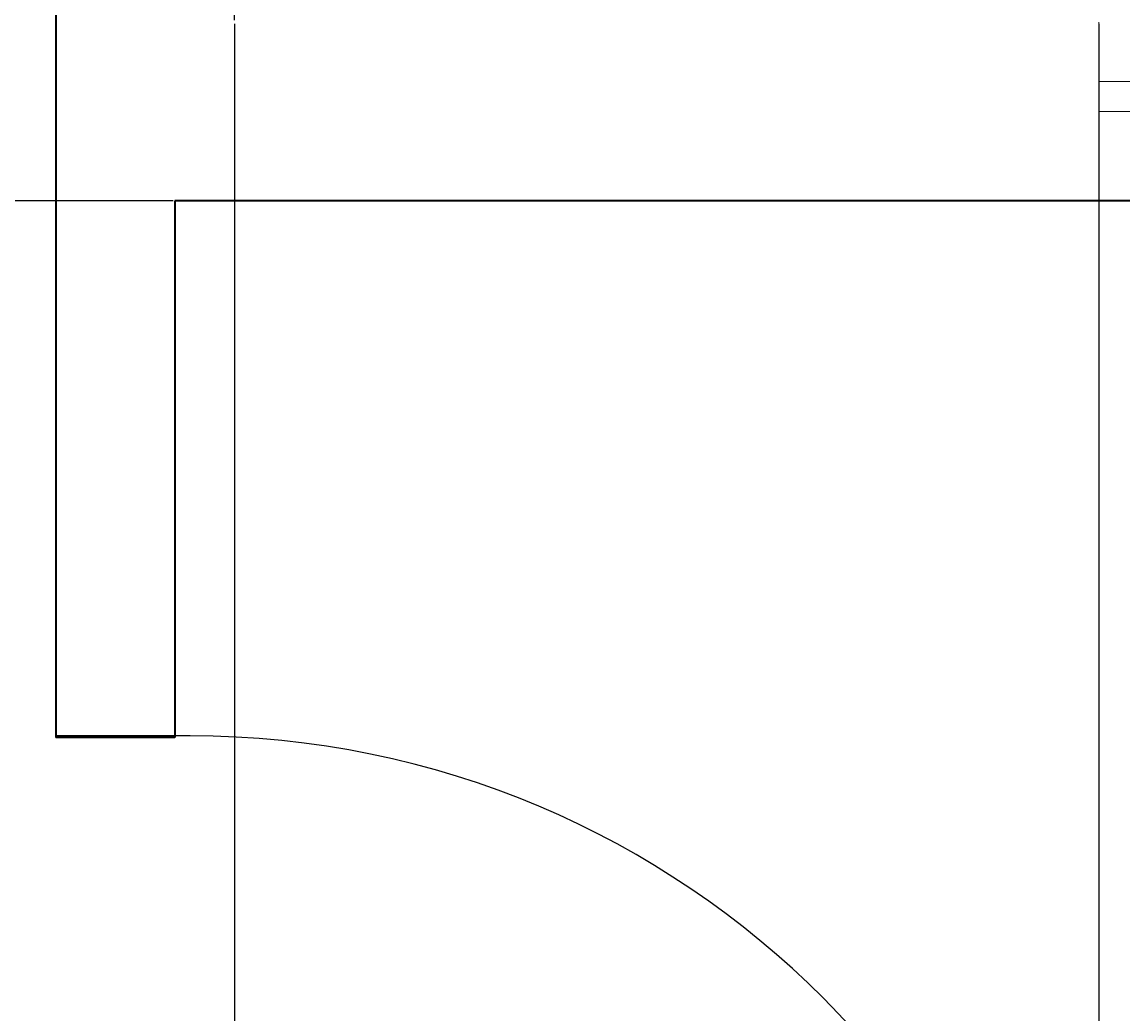
# Model space of a CAD drawing. Units: feet. Extents: x 105 to 1094, y -88 to 588.
# Tile 8 of 59: x 288 to 324, y 171 to 204. Entities that reach past the tile are written whole.
import ezdxf

# ---------------------------------------------------------------- set-up
doc = ezdxf.new("R2010")
doc.units = ezdxf.units.FT
doc.header["$MEASUREMENT"] = 0
for name, color, linetype, lineweight in [('A-ANNO-DIMS', 2, 'Continuous', 18), ('A-DOOR', 3, 'Continuous', 25), ('A-GLAZ', 4, 'Continuous', 18), ('A-WALL', 7, 'Continuous', 35)]:
    doc.layers.add(name, color=color, linetype=linetype, lineweight=lineweight)
doc.styles.get("Standard").update_dxf_attribs({"font": 'arial.ttf'})
doc.dimstyles.get("Standard").update_dxf_attribs({"dimtxt": 0.18, "dimasz": 0.18, "dimexe": 0.18, "dimexo": 0.0625, "dimgap": 0.09, "dimtad": 0, "dimtih": 1, "dimtoh": 1, "dimdec": 4, "dimzin": 0, "dimdsep": 46, "dimtxsty": 'Standard', "dimcen": 0.09, "dimadec": 0, "dimazin": 0, "dimtfac": 1, "dimtdec": 4, "dimtofl": 0, "dimtmove": 0, "dimatfit": 3, "dimfxl": 1, "dimtolj": 1, "dimtzin": 0, "dimarcsym": 0})

# ---------------------------------------------------------------- blocks, each defined once
blk = doc.blocks.new('*U4')
for p, q in [((0, 0), (0, -6)), ((-40, 0), (-40, -6))]:
    blk.add_line(p, q)
blk.add_lwpolyline([(0, 0), (0, 40), (-1.75, 40), (-1.75, 0)], close=True)
blk.add_arc((0, 0), 40, 90, 180)
blk = doc.blocks.new('VENT-TRANSVERSE')
for p, q in [((0, 0), (0, 6)), ((18, 0), (18, 6)), ((0, 3), (18, 3)), ((0, 2), (18, 2))]:
    blk.add_line(p, q)
blk = doc.blocks.new('*D20')
at = {"layer": 'A-ANNO-DIMS', "color": 0, "lineweight": -2, "transparency": 16777216}
for p, q in [((150.688, 276.019), (150.688, -88.149)), ((1048.688, 276.019), (1048.688, -88.149)), ((150.868, -87.969), (599.399, -87.969)), ((1048.508, -87.969), (599.977, -87.969))]:
    blk.add_line(p, q, dxfattribs=at)
at = {"layer": 'A-ANNO-DIMS', "color": 0, "transparency": 16777216}
for points in [[(150.868, -87.939), (150.868, -87.999), (150.688, -87.969)], [(1048.508, -87.939), (1048.508, -87.999), (1048.688, -87.969)]]:
    blk.add_solid(points, dxfattribs=at)
at = {"layer": 'Defpoints', "color": 0, "transparency": 16777216}
for p in [(150.688, 276.081), (1048.688, 276.081), (1048.688, -87.969)]:
    blk.add_point(p, dxfattribs=at)
at = {"layer": 'A-ANNO-DIMS', "color": 0, "transparency": 16777216, "insert": (599.688, -87.969), "char_height": 0.18, "attachment_point": 5}
blk.add_mtext('\\A1;898', dxfattribs=at)
blk = doc.blocks.new('*D21')
at = {"layer": 'A-ANNO-DIMS', "color": 0, "lineweight": -2, "transparency": 16777216}
for p, q in [((849.626, 543.081), (105.458, 543.081)), ((105.638, 542.901), (105.638, 250.263)), ((105.638, -42.739), (105.638, 249.899)), ((849.626, -42.919), (105.458, -42.919))]:
    blk.add_line(p, q, dxfattribs=at)
at = {"layer": 'A-ANNO-DIMS', "color": 0, "transparency": 16777216}
for points in [[(105.608, 542.901), (105.668, 542.901), (105.638, 543.081)], [(105.608, -42.739), (105.668, -42.739), (105.638, -42.919)]]:
    blk.add_solid(points, dxfattribs=at)
at = {"layer": 'Defpoints', "color": 0, "transparency": 16777216}
for p in [(105.638, 543.081), (849.688, 543.081), (849.688, -42.919)]:
    blk.add_point(p, dxfattribs=at)
at = {"layer": 'A-ANNO-DIMS', "color": 0, "transparency": 16777216, "insert": (105.638, 250.081), "char_height": 0.18, "attachment_point": 5}
blk.add_mtext('\\A1;586', dxfattribs=at)
blk = doc.blocks.new('*D39')
at = {"layer": 'A-ANNO-DIMS', "color": 0, "lineweight": -2, "transparency": 16777216}
for p, q in [((294.688, 204.144), (294.688, 588.311)), ((294.868, 588.131), (332.47, 588.131)), ((370.508, 588.131), (332.906, 588.131)), ((370.688, 204.144), (370.688, 588.311))]:
    blk.add_line(p, q, dxfattribs=at)
at = {"layer": 'A-ANNO-DIMS', "color": 0, "transparency": 16777216}
for points in [[(294.868, 588.161), (294.868, 588.101), (294.688, 588.131)], [(370.508, 588.161), (370.508, 588.101), (370.688, 588.131)]]:
    blk.add_solid(points, dxfattribs=at)
at = {"layer": 'Defpoints', "color": 0, "transparency": 16777216}
for p in [(370.688, 588.131), (294.688, 204.081), (370.688, 204.081)]:
    blk.add_point(p, dxfattribs=at)
at = {"layer": 'A-ANNO-DIMS', "color": 0, "transparency": 16777216, "insert": (332.688, 588.131), "char_height": 0.18, "attachment_point": 5}
blk.add_mtext('\\A1;76', dxfattribs=at)
blk = doc.blocks.new('*D44')
at = {"layer": 'A-ANNO-DIMS', "color": 0, "lineweight": -2, "transparency": 16777216}
for p, q in [((294.688, 204.019), (294.688, -88.149)), ((323.688, 204.019), (323.688, -88.149)), ((294.868, -87.969), (308.968, -87.969)), ((323.508, -87.969), (309.409, -87.969))]:
    blk.add_line(p, q, dxfattribs=at)
at = {"layer": 'A-ANNO-DIMS', "color": 0, "transparency": 16777216}
for points in [[(294.868, -87.939), (294.868, -87.999), (294.688, -87.969)], [(323.508, -87.939), (323.508, -87.999), (323.688, -87.969)]]:
    blk.add_solid(points, dxfattribs=at)
at = {"layer": 'Defpoints', "color": 0, "transparency": 16777216}
for p in [(294.688, 204.081), (323.688, 204.081), (323.688, -87.969)]:
    blk.add_point(p, dxfattribs=at)
at = {"layer": 'A-ANNO-DIMS', "color": 0, "transparency": 16777216, "insert": (309.188, -87.969), "char_height": 0.18, "attachment_point": 5}
blk.add_mtext('\\A1;29', dxfattribs=at)
blk = doc.blocks.new('*D46')
at = {"layer": 'A-ANNO-DIMS', "color": 0, "lineweight": -2, "transparency": 16777216}
for p, q in [((580.626, 206.081), (105.458, 206.081)), ((105.638, 205.901), (105.638, 173.263)), ((105.638, 140.261), (105.638, 172.899)), ((580.626, 140.081), (105.458, 140.081))]:
    blk.add_line(p, q, dxfattribs=at)
at = {"layer": 'A-ANNO-DIMS', "color": 0, "transparency": 16777216}
for points in [[(105.608, 205.901), (105.668, 205.901), (105.638, 206.081)], [(105.608, 140.261), (105.668, 140.261), (105.638, 140.081)]]:
    blk.add_solid(points, dxfattribs=at)
at = {"layer": 'Defpoints', "color": 0, "transparency": 16777216}
for p in [(580.688, 206.081), (105.638, 140.081), (580.688, 140.081)]:
    blk.add_point(p, dxfattribs=at)
at = {"layer": 'A-ANNO-DIMS', "color": 0, "transparency": 16777216, "insert": (105.638, 173.081), "char_height": 0.18, "attachment_point": 5}
blk.add_mtext('\\A1;66', dxfattribs=at)
blk = doc.blocks.new('*D55')
at = {"layer": 'A-ANNO-DIMS', "color": 0, "lineweight": -2, "transparency": 16777216}
for p, q in [((292.626, 198.081), (105.458, 198.081)), ((105.638, 197.901), (105.638, 174.263)), ((105.638, 150.261), (105.638, 173.899)), ((293.134, 150.081), (105.458, 150.081))]:
    blk.add_line(p, q, dxfattribs=at)
at = {"layer": 'A-ANNO-DIMS', "color": 0, "transparency": 16777216}
for points in [[(105.608, 197.901), (105.668, 197.901), (105.638, 198.081)], [(105.608, 150.261), (105.668, 150.261), (105.638, 150.081)]]:
    blk.add_solid(points, dxfattribs=at)
at = {"layer": 'Defpoints', "color": 0, "transparency": 16777216}
for p in [(105.638, 198.081), (292.688, 198.081), (293.197, 150.081)]:
    blk.add_point(p, dxfattribs=at)
at = {"layer": 'A-ANNO-DIMS', "color": 0, "transparency": 16777216, "insert": (105.638, 174.081), "char_height": 0.18, "attachment_point": 5}
blk.add_mtext('\\A1;48', dxfattribs=at)

msp = doc.modelspace()

# ---------------------------------------------------------------- linework, layer by layer
at = {"layer": 'A-WALL'}
for p, q in [((288.6883, 218.0812), (288.6883, 180.0812)), ((370.6883, 198.0812), (292.6883, 198.0812)), ((292.6883, 198.0812), (292.6883, 180.0812)), ((292.6883, 180.0812), (288.6883, 180.0812))]:
    msp.add_line(p, q, dxfattribs=at)

# ---------------------------------------------------------------- block references
at = {"layer": 'A-DOOR', "xscale": 0.7513941790917756, "yscale": 0.7513941790917756, "zscale": 0.7513941790917756, "rotation": 270}
msp.add_blockref('*U4', (293.1967, 150.0812), dxfattribs=at)
at = {"layer": 'A-GLAZ', "rotation": 180}
msp.add_blockref('VENT-TRANSVERSE', (341.6886, 204.0813), dxfattribs=at)

# ---------------------------------------------------------------- dimensions: what is measured, and where the dimension line sits
at = {"layer": 'A-ANNO-DIMS'}
for base, p1, p2, picture, middle in [((370.6883, 588.1312), (294.6883, 204.0812), (370.6883, 204.0812), '*D39', (332.6883, 588.1312)), ((1048.6883, -87.9688), (150.6883, 276.0812), (1048.6883, 276.0812), '*D20', (599.6883, -87.9688)), ((323.6883, -87.9688), (294.6883, 204.0812), (323.6883, 204.0812), '*D44', (309.1883, -87.9688))]:
    dim = msp.add_linear_dim(base=base, p1=p1, p2=p2, dimstyle='Standard', override={"dimdec": 0, "dimlfac": 1, "dimrnd": 0, "dimzin": 0, "dimdsep": 46, "dimlunit": 2}, dxfattribs=at)
    dim.commit()
    dim.dimension.update_dxf_attribs({"geometry": picture, "text_midpoint": middle})
for base, p1, p2, picture, middle in [((105.6383, 543.0812), (849.6883, -42.9188), (849.6883, 543.0812), '*D21', (105.6383, 250.0812)), ((105.6383, 140.0812), (580.6883, 206.0812), (580.6883, 140.0812), '*D46', (105.6383, 173.0812)), ((105.6383, 198.0812), (293.1967, 150.0812), (292.6883, 198.0812), '*D55', (105.6383, 174.0812))]:
    dim = msp.add_linear_dim(base=base, p1=p1, p2=p2, angle=90, dimstyle='Standard', override={"dimdec": 0, "dimlfac": 1, "dimrnd": 0, "dimzin": 0, "dimdsep": 46, "dimlunit": 2}, dxfattribs=at)
    dim.commit()
    dim.dimension.update_dxf_attribs({"geometry": picture, "text_midpoint": middle})

doc.saveas('drawing.dxf')
